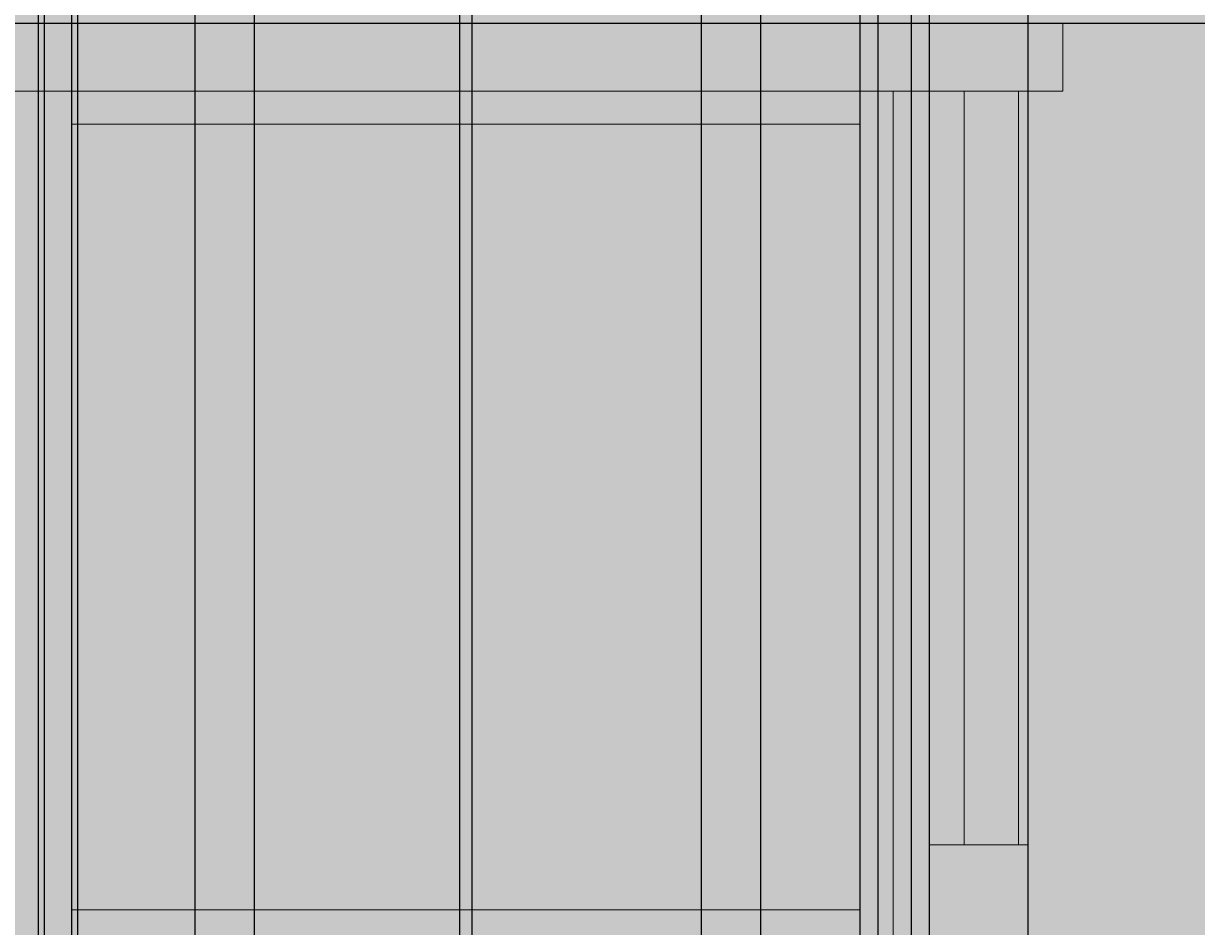
# Model space of a CAD drawing. Units: inches. Extents: x 3024 to 4744, y 1110 to 2100.
# Tile 9 of 29: x 3168 to 3309, y 1293 to 1402. Entities that reach past the tile are written whole.
import ezdxf

# ---------------------------------------------------------------- set-up
doc = ezdxf.new("R2010")
doc.units = ezdxf.units.IN
for name, color, linetype, lineweight in [('A-ANNO-DIMS', 2, 'Continuous', 18), ('A-ELEV', 7, 'Continuous', 25), ('A-ELEV-PATT', 252, 'Continuous', 13), ('A-GLAZ', 4, 'Continuous', 18)]:
    doc.layers.add(name, color=color, linetype=linetype, lineweight=lineweight)
doc.styles.get("Standard").update_dxf_attribs({"font": 'arial.ttf'})
doc.dimstyles.get("Standard").update_dxf_attribs({"dimtxt": 0.18, "dimasz": 0.18, "dimexe": 0.18, "dimexo": 0.0625, "dimgap": 0.09, "dimtad": 0, "dimtih": 1, "dimtoh": 1, "dimdec": 1, "dimzin": 0, "dimdsep": 46, "dimlunit": 3, "dimtxsty": 'Standard', "dimcen": 0.09, "dimadec": 0, "dimazin": 0, "dimtfac": 1, "dimtdec": 1, "dimtofl": 0, "dimtmove": 0, "dimatfit": 3, "dimfxl": 1, "dimtolj": 1, "dimtzin": 0, "dimarcsym": 0})

# ---------------------------------------------------------------- blocks, each defined once
blk = doc.blocks.new('WIN-BALCONY-A')
for q in [(3148.97, 1897.49), (3148.97, 1897.49), (3292.61, 1897.49), (3292.61, 1897.49)]:
    blk.add_line((3169.4, 1897.49), q)
blk.add_lwpolyline([(3148.97, 1897.49), (3148.97, 1905.61), (3292.61, 1905.61), (3292.61, 1897.49)])
blk.add_lwpolyline([(3148.97, 1897.49), (3148.97, 1905.61), (3292.61, 1905.61), (3292.61, 1897.49)])
for points in [[(3272.18, 1795.04), (3169.4, 1795.04), (3169.4, 1897.49), (3272.18, 1897.49)], [(3272.18, 1795.04), (3169.4, 1795.04), (3169.4, 1897.49), (3272.18, 1897.49)], [(3287.25, 1806.87), (3280.72, 1806.87), (3280.72, 1897.49), (3287.25, 1897.49)], [(3287.25, 1806.87), (3280.72, 1806.87), (3280.72, 1897.49), (3287.25, 1897.49)], [(3268.18, 1799.04), (3173.4, 1799.04), (3173.4, 1893.49), (3268.18, 1893.49)], [(3268.18, 1799.04), (3173.4, 1799.04), (3173.4, 1893.49), (3268.18, 1893.49)], [(3220.05, 1893.49), (3221.52, 1893.49), (3221.52, 1799.04), (3220.05, 1799.04)], [(3220.05, 1893.49), (3221.52, 1893.49), (3221.52, 1799.04), (3220.05, 1799.04)], [(3276.51, 1795.04), (3288.38, 1795.04), (3288.38, 1806.87), (3276.51, 1806.87)], [(3276.51, 1795.04), (3288.38, 1795.04), (3288.38, 1806.87), (3276.51, 1806.87)]]:
    blk.add_lwpolyline(points, close=True)
blk = doc.blocks.new('*D64')
at = {"layer": 'A-ANNO-DIMS', "color": 0, "lineweight": -2, "transparency": 16777216}
for p, q in [((3069.79, 1241.5), (3069.79, 2100.44)), ((3069.97, 2100.26), (3405.08, 2100.26)), ((3740.97, 2100.26), (3405.87, 2100.26)), ((3741.15, 1241.5), (3741.15, 2100.44))]:
    blk.add_line(p, q, dxfattribs=at)
at = {"layer": 'A-ANNO-DIMS', "color": 0, "transparency": 16777216}
for points in [[(3069.97, 2100.29), (3069.97, 2100.23), (3069.79, 2100.26)], [(3740.97, 2100.29), (3740.97, 2100.23), (3741.15, 2100.26)]]:
    blk.add_solid(points, dxfattribs=at)
at = {"layer": 'Defpoints', "color": 0, "transparency": 16777216}
for p in [(3741.15, 2100.26), (3069.79, 1241.43), (3741.15, 1241.43)]:
    blk.add_point(p, dxfattribs=at)
at = {"layer": 'A-ANNO-DIMS', "color": 0, "transparency": 16777216, "insert": (3405.47, 2100.26), "char_height": 0.18, "attachment_point": 5}
blk.add_mtext('\\A1;671.4', dxfattribs=at)
blk = doc.blocks.new('*D90')
at = {"layer": 'A-ANNO-DIMS', "color": 0, "lineweight": -2, "transparency": 16777216}
for p, q in [((3173.4, 1798.98), (3173.4, 1109.93)), ((3169.4, 1794.98), (3169.4, 1109.93)), ((3169.58, 1110.11), (3171.07, 1110.11)), ((3173.22, 1110.11), (3171.72, 1110.11))]:
    blk.add_line(p, q, dxfattribs=at)
at = {"layer": 'A-ANNO-DIMS', "color": 0, "transparency": 16777216}
for points in [[(3169.58, 1110.14), (3169.58, 1110.08), (3169.4, 1110.11)], [(3173.22, 1110.14), (3173.22, 1110.08), (3173.4, 1110.11)]]:
    blk.add_solid(points, dxfattribs=at)
at = {"layer": 'Defpoints', "color": 0, "transparency": 16777216}
for p in [(3173.4, 1799.04), (3169.4, 1795.04), (3173.4, 1110.11)]:
    blk.add_point(p, dxfattribs=at)
at = {"layer": 'A-ANNO-DIMS', "color": 0, "transparency": 16777216, "insert": (3171.4, 1110.11), "char_height": 0.18, "attachment_point": 5}
blk.add_mtext('\\A1;4.00', dxfattribs=at)
blk = doc.blocks.new('*D91')
at = {"layer": 'A-ANNO-DIMS', "color": 0, "lineweight": -2, "transparency": 16777216}
for p, q in [((3173.4, 1798.98), (3173.4, 1109.93)), ((3220.05, 1798.98), (3220.05, 1109.93)), ((3173.58, 1110.11), (3196.33, 1110.11)), ((3219.87, 1110.11), (3197.12, 1110.11))]:
    blk.add_line(p, q, dxfattribs=at)
at = {"layer": 'A-ANNO-DIMS', "color": 0, "transparency": 16777216}
for points in [[(3173.58, 1110.14), (3173.58, 1110.08), (3173.4, 1110.11)], [(3219.87, 1110.14), (3219.87, 1110.08), (3220.05, 1110.11)]]:
    blk.add_solid(points, dxfattribs=at)
at = {"layer": 'Defpoints', "color": 0, "transparency": 16777216}
for p in [(3173.4, 1799.04), (3220.05, 1799.04), (3220.05, 1110.11)]:
    blk.add_point(p, dxfattribs=at)
at = {"layer": 'A-ANNO-DIMS', "color": 0, "transparency": 16777216, "insert": (3196.72, 1110.11), "char_height": 0.18, "attachment_point": 5}
blk.add_mtext('\\A1;46.65', dxfattribs=at)
blk = doc.blocks.new('*D92')
at = {"layer": 'A-ANNO-DIMS', "color": 0, "lineweight": -2, "transparency": 16777216}
for p, q in [((3220.05, 1798.98), (3220.05, 1109.93)), ((3221.52, 1798.98), (3221.52, 1109.93)), ((3220.23, 1110.11), (3220.47, 1110.11)), ((3221.34, 1110.11), (3221.1, 1110.11))]:
    blk.add_line(p, q, dxfattribs=at)
at = {"layer": 'A-ANNO-DIMS', "color": 0, "transparency": 16777216}
for points in [[(3220.23, 1110.14), (3220.23, 1110.08), (3220.05, 1110.11)], [(3221.34, 1110.14), (3221.34, 1110.08), (3221.52, 1110.11)]]:
    blk.add_solid(points, dxfattribs=at)
at = {"layer": 'Defpoints', "color": 0, "transparency": 16777216}
for p in [(3220.05, 1799.04), (3221.52, 1799.04), (3221.52, 1110.11)]:
    blk.add_point(p, dxfattribs=at)
at = {"layer": 'A-ANNO-DIMS', "color": 0, "transparency": 16777216, "insert": (3220.79, 1110.11), "char_height": 0.18, "attachment_point": 5}
blk.add_mtext('\\A1;1.47', dxfattribs=at)
blk = doc.blocks.new('*D93')
at = {"layer": 'A-ANNO-DIMS', "color": 0, "lineweight": -2, "transparency": 16777216}
for p, q in [((3221.52, 1798.98), (3221.52, 1109.93)), ((3268.18, 1798.98), (3268.18, 1109.93)), ((3221.7, 1110.11), (3244.45, 1110.11)), ((3268, 1110.11), (3245.25, 1110.11))]:
    blk.add_line(p, q, dxfattribs=at)
at = {"layer": 'A-ANNO-DIMS', "color": 0, "transparency": 16777216}
for points in [[(3221.7, 1110.14), (3221.7, 1110.08), (3221.52, 1110.11)], [(3268, 1110.14), (3268, 1110.08), (3268.18, 1110.11)]]:
    blk.add_solid(points, dxfattribs=at)
at = {"layer": 'Defpoints', "color": 0, "transparency": 16777216}
for p in [(3221.52, 1799.04), (3268.18, 1799.04), (3268.18, 1110.11)]:
    blk.add_point(p, dxfattribs=at)
at = {"layer": 'A-ANNO-DIMS', "color": 0, "transparency": 16777216, "insert": (3244.85, 1110.11), "char_height": 0.18, "attachment_point": 5}
blk.add_mtext('\\A1;46.65', dxfattribs=at)
blk = doc.blocks.new('*D94')
at = {"layer": 'A-ANNO-DIMS', "color": 0, "lineweight": -2, "transparency": 16777216}
for p, q in [((3276.51, 1794.98), (3276.51, 1109.93)), ((3288.38, 1794.98), (3288.38, 1109.93)), ((3276.69, 1110.11), (3281.99, 1110.11)), ((3288.2, 1110.11), (3282.9, 1110.11))]:
    blk.add_line(p, q, dxfattribs=at)
at = {"layer": 'A-ANNO-DIMS', "color": 0, "transparency": 16777216}
for points in [[(3276.69, 1110.14), (3276.69, 1110.08), (3276.51, 1110.11)], [(3288.2, 1110.14), (3288.2, 1110.08), (3288.38, 1110.11)]]:
    blk.add_solid(points, dxfattribs=at)
at = {"layer": 'Defpoints', "color": 0, "transparency": 16777216}
for p in [(3276.51, 1795.04), (3288.38, 1795.04), (3288.38, 1110.11)]:
    blk.add_point(p, dxfattribs=at)
at = {"layer": 'A-ANNO-DIMS', "color": 0, "transparency": 16777216, "insert": (3282.44, 1110.11), "char_height": 0.18, "attachment_point": 5}
blk.add_mtext('\\A1;11.866', dxfattribs=at)
blk = doc.blocks.new('*D106')
at = {"layer": 'A-ANNO-DIMS', "color": 0, "lineweight": -2, "transparency": 16777216}
for p, q in [((3170.16, 1275.67), (3170.16, 2100.44)), ((3170.34, 2100.26), (3171.83, 2100.26)), ((3173.98, 2100.26), (3172.49, 2100.26)), ((3174.16, 1271.67), (3174.16, 2100.44))]:
    blk.add_line(p, q, dxfattribs=at)
at = {"layer": 'A-ANNO-DIMS', "color": 0, "transparency": 16777216}
for points in [[(3170.34, 2100.29), (3170.34, 2100.23), (3170.16, 2100.26)], [(3173.98, 2100.29), (3173.98, 2100.23), (3174.16, 2100.26)]]:
    blk.add_solid(points, dxfattribs=at)
at = {"layer": 'Defpoints', "color": 0, "transparency": 16777216}
for p in [(3174.16, 2100.26), (3170.16, 1275.61), (3174.16, 1271.61)]:
    blk.add_point(p, dxfattribs=at)
at = {"layer": 'A-ANNO-DIMS', "color": 0, "transparency": 16777216, "insert": (3172.16, 2100.26), "char_height": 0.18, "attachment_point": 5}
blk.add_mtext('\\A1;4.00', dxfattribs=at)
blk = doc.blocks.new('*D107')
at = {"layer": 'A-ANNO-DIMS', "color": 0, "lineweight": -2, "transparency": 16777216}
for p, q in [((3174.16, 1271.67), (3174.16, 2100.44)), ((3174.34, 2100.26), (3221.88, 2100.26)), ((3270.21, 2100.26), (3222.67, 2100.26)), ((3270.39, 1271.67), (3270.39, 2100.44))]:
    blk.add_line(p, q, dxfattribs=at)
at = {"layer": 'A-ANNO-DIMS', "color": 0, "transparency": 16777216}
for points in [[(3174.34, 2100.29), (3174.34, 2100.23), (3174.16, 2100.26)], [(3270.21, 2100.29), (3270.21, 2100.23), (3270.39, 2100.26)]]:
    blk.add_solid(points, dxfattribs=at)
at = {"layer": 'Defpoints', "color": 0, "transparency": 16777216}
for p in [(3270.39, 2100.26), (3174.16, 1271.61), (3270.39, 1271.61)]:
    blk.add_point(p, dxfattribs=at)
at = {"layer": 'A-ANNO-DIMS', "color": 0, "transparency": 16777216, "insert": (3222.27, 2100.26), "char_height": 0.18, "attachment_point": 5}
blk.add_mtext('\\A1;96.23', dxfattribs=at)
blk = doc.blocks.new('*D108')
at = {"layer": 'A-ANNO-DIMS', "color": 0, "lineweight": -2, "transparency": 16777216}
for p, q in [((3270.39, 1271.67), (3270.39, 2100.44)), ((3270.57, 2100.26), (3272.06, 2100.26)), ((3274.21, 2100.26), (3272.71, 2100.26)), ((3274.39, 1275.67), (3274.39, 2100.44))]:
    blk.add_line(p, q, dxfattribs=at)
at = {"layer": 'A-ANNO-DIMS', "color": 0, "transparency": 16777216}
for points in [[(3270.57, 2100.29), (3270.57, 2100.23), (3270.39, 2100.26)], [(3274.21, 2100.29), (3274.21, 2100.23), (3274.39, 2100.26)]]:
    blk.add_solid(points, dxfattribs=at)
at = {"layer": 'Defpoints', "color": 0, "transparency": 16777216}
for p in [(3274.39, 2100.26), (3274.39, 1275.61), (3270.39, 1271.61)]:
    blk.add_point(p, dxfattribs=at)
at = {"layer": 'A-ANNO-DIMS', "color": 0, "transparency": 16777216, "insert": (3272.39, 2100.26), "char_height": 0.18, "attachment_point": 5}
blk.add_mtext('\\A1;4.00', dxfattribs=at)
blk = doc.blocks.new('*D124')
at = {"layer": 'A-ANNO-DIMS', "color": 0, "lineweight": -2, "transparency": 16777216}
for p, q in [((3174.16, 1271.67), (3174.16, 2100.44)), ((3174.34, 2100.26), (3180.75, 2100.26)), ((3188.08, 2100.26), (3181.67, 2100.26)), ((3188.26, 1256.29), (3188.26, 2100.44))]:
    blk.add_line(p, q, dxfattribs=at)
at = {"layer": 'A-ANNO-DIMS', "color": 0, "transparency": 16777216}
for points in [[(3174.34, 2100.29), (3174.34, 2100.23), (3174.16, 2100.26)], [(3188.08, 2100.29), (3188.08, 2100.23), (3188.26, 2100.26)]]:
    blk.add_solid(points, dxfattribs=at)
at = {"layer": 'Defpoints', "color": 0, "transparency": 16777216}
for p in [(3188.26, 2100.26), (3174.16, 1271.61), (3188.26, 1256.23)]:
    blk.add_point(p, dxfattribs=at)
at = {"layer": 'A-ANNO-DIMS', "color": 0, "transparency": 16777216, "insert": (3181.21, 2100.26), "char_height": 0.18, "attachment_point": 5}
blk.add_mtext('\\A1;14.098', dxfattribs=at)
blk = doc.blocks.new('*D125')
at = {"layer": 'A-ANNO-DIMS', "color": 0, "lineweight": -2, "transparency": 16777216}
for p, q in [((3188.26, 1256.29), (3188.26, 2100.44)), ((3188.44, 2100.26), (3191.44, 2100.26)), ((3195.23, 2100.26), (3192.22, 2100.26)), ((3195.41, 1256.29), (3195.41, 2100.44))]:
    blk.add_line(p, q, dxfattribs=at)
at = {"layer": 'A-ANNO-DIMS', "color": 0, "transparency": 16777216}
for points in [[(3188.44, 2100.29), (3188.44, 2100.23), (3188.26, 2100.26)], [(3195.23, 2100.29), (3195.23, 2100.23), (3195.41, 2100.26)]]:
    blk.add_solid(points, dxfattribs=at)
at = {"layer": 'Defpoints', "color": 0, "transparency": 16777216}
for p in [(3195.41, 2100.26), (3188.26, 1256.23), (3195.41, 1256.23)]:
    blk.add_point(p, dxfattribs=at)
at = {"layer": 'A-ANNO-DIMS', "color": 0, "transparency": 16777216, "insert": (3191.83, 2100.26), "char_height": 0.18, "attachment_point": 5}
blk.add_mtext('\\A1;7.147', dxfattribs=at)
blk = doc.blocks.new('*D126')
at = {"layer": 'A-ANNO-DIMS', "color": 0, "lineweight": -2, "transparency": 16777216}
for p, q in [((3249.14, 1256.29), (3249.14, 2100.44)), ((3249.32, 2100.26), (3252.32, 2100.26)), ((3256.11, 2100.26), (3253.11, 2100.26)), ((3256.29, 1256.29), (3256.29, 2100.44))]:
    blk.add_line(p, q, dxfattribs=at)
at = {"layer": 'A-ANNO-DIMS', "color": 0, "transparency": 16777216}
for points in [[(3249.32, 2100.29), (3249.32, 2100.23), (3249.14, 2100.26)], [(3256.11, 2100.29), (3256.11, 2100.23), (3256.29, 2100.26)]]:
    blk.add_solid(points, dxfattribs=at)
at = {"layer": 'Defpoints', "color": 0, "transparency": 16777216}
for p in [(3256.29, 2100.26), (3249.14, 1256.23), (3256.29, 1256.23)]:
    blk.add_point(p, dxfattribs=at)
at = {"layer": 'A-ANNO-DIMS', "color": 0, "transparency": 16777216, "insert": (3252.72, 2100.26), "char_height": 0.18, "attachment_point": 5}
blk.add_mtext('\\A1;7.147', dxfattribs=at)

msp = doc.modelspace()

# ---------------------------------------------------------------- hatches: boundary and pattern name
at = {"layer": 'A-ELEV-PATT'}
h = msp.add_hatch(color=256, dxfattribs=at)
h.dxf.hatch_style = 1
h.paths.add_polyline_path([(3491.8271, 2054.7584), (3320.5658, 2054.7584), (3320.5658, 2043.5286), (3491.8271, 2043.5286)])
h.paths.add_polyline_path([(3292.6051, 1905.6112), (3148.9694, 1905.6112), (3148.9694, 1897.4879), (3169.3964, 1897.4879), (3292.6051, 1897.4879)])
h.paths.add_polyline_path([(3292.6051, 1795.0431), (3169.3964, 1795.0431), (3148.9694, 1795.0431), (3148.9694, 1785.6112), (3292.6051, 1785.6112)])
h.paths.add_polyline_path([(3292.6051, 1779.6112), (3148.9694, 1779.6112), (3148.9694, 1771.4879), (3169.3964, 1771.4879), (3292.6051, 1771.4879)])
h.paths.add_polyline_path([(3292.6051, 1669.0431), (3169.3964, 1669.0431), (3148.9694, 1669.0431), (3148.9694, 1659.6112), (3292.6051, 1659.6112)])
h.paths.add_polyline_path([(3292.6051, 1653.6112), (3148.9694, 1653.6112), (3148.9694, 1645.4879), (3169.3964, 1645.4879), (3292.6051, 1645.4879)])
h.paths.add_polyline_path([(3292.6051, 1543.0431), (3169.3964, 1543.0431), (3148.9694, 1543.0431), (3148.9694, 1533.6112), (3292.6051, 1533.6112)])
h.paths.add_polyline_path([(3292.6051, 1527.6112), (3148.9694, 1527.6112), (3148.9694, 1519.4879), (3169.3964, 1519.4879), (3292.6051, 1519.4879)])
h.paths.add_polyline_path([(3292.6051, 1401.6112), (3148.9694, 1401.6112), (3148.9694, 1393.4879), (3169.3964, 1393.4879), (3292.6051, 1393.4879)])
h.paths.add_polyline_path([(3292.6051, 1417.0431), (3169.3964, 1417.0431), (3148.9694, 1417.0431), (3148.9694, 1407.6112), (3292.6051, 1407.6112)])
h.paths.add_polyline_path([(3292.6051, 1291.0431), (3169.3964, 1291.0431), (3148.9694, 1291.0431), (3148.9694, 1281.6112), (3292.6051, 1281.6112)])
h.paths.add_polyline_path([(3654.037, 1165.0431), (3530.8283, 1165.0431), (3510.4013, 1165.0431), (3510.4013, 1155.6112), (3654.037, 1155.6112)])
h.paths.add_polyline_path([(3654.037, 1275.6112), (3510.4013, 1275.6112), (3510.4013, 1267.4879), (3530.8283, 1267.4879), (3654.037, 1267.4879)])
h.paths.add_polyline_path([(3654.037, 1291.0431), (3530.8283, 1291.0431), (3510.4013, 1291.0431), (3510.4013, 1281.6112), (3654.037, 1281.6112)])
h.paths.add_polyline_path([(3654.037, 1417.0431), (3530.8283, 1417.0431), (3510.4013, 1417.0431), (3510.4013, 1407.6112), (3654.037, 1407.6112)])
h.paths.add_polyline_path([(3654.037, 1401.6112), (3510.4013, 1401.6112), (3510.4013, 1393.4879), (3530.8283, 1393.4879), (3654.037, 1393.4879)])
h.paths.add_polyline_path([(3654.037, 1543.0431), (3530.8283, 1543.0431), (3510.4013, 1543.0431), (3510.4013, 1533.6112), (3654.037, 1533.6112)])
h.paths.add_polyline_path([(3654.037, 1527.6112), (3510.4013, 1527.6112), (3510.4013, 1519.4879), (3530.8283, 1519.4879), (3654.037, 1519.4879)])
h.paths.add_polyline_path([(3654.037, 1653.6112), (3510.4013, 1653.6112), (3510.4013, 1645.4879), (3530.8283, 1645.4879), (3654.037, 1645.4879)])
h.paths.add_polyline_path([(3654.037, 1669.0431), (3530.8283, 1669.0431), (3510.4013, 1669.0431), (3510.4013, 1659.6112), (3654.037, 1659.6112)])
h.paths.add_polyline_path([(3654.037, 1779.6112), (3510.4013, 1779.6112), (3510.4013, 1771.4879), (3530.8283, 1771.4879), (3654.037, 1771.4879)])
h.paths.add_polyline_path([(3654.037, 1795.0431), (3530.8283, 1795.0431), (3510.4013, 1795.0431), (3510.4013, 1785.6112), (3654.037, 1785.6112)])
h.paths.add_polyline_path([(3654.037, 1905.6112), (3510.4013, 1905.6112), (3510.4013, 1897.4879), (3530.8283, 1897.4879), (3654.037, 1897.4879)])
h = msp.add_hatch(color=256, dxfattribs=at)
h.dxf.hatch_style = 1
h.paths.add_polyline_path([(3329.7033, 1407.6112), (3105.4722, 1407.6112), (3105.4722, 1401.6112), (3329.7033, 1401.6112)])
h.paths.add_polyline_path([(3329.7033, 1281.6112), (3105.4722, 1281.6112), (3105.4722, 1275.6112), (3112.3838, 1275.6112), (3329.7033, 1275.6112)])
h.paths.add_polyline_path([(3329.7033, 1533.6112), (3105.4722, 1533.6112), (3105.4722, 1527.6112), (3329.7033, 1527.6112)])
h.paths.add_polyline_path([(3329.7033, 1659.6112), (3105.4722, 1659.6112), (3105.4722, 1653.6112), (3329.7033, 1653.6112)])
h.paths.add_polyline_path([(3329.7033, 1785.6112), (3105.4722, 1785.6112), (3105.4722, 1779.6112), (3329.7033, 1779.6112)])
h.paths.add_polyline_path([(3329.7033, 1911.6112), (3105.4722, 1911.6112), (3095.7158, 1911.6112), (3095.7158, 1905.6112), (3329.7033, 1905.6112)])
h.paths.add_polyline_path([(3715.2286, 1911.6112), (3705.4722, 1911.6112), (3705.4722, 1905.6112), (3715.2286, 1905.6112)])
h.paths.add_polyline_path([(3688.5588, 1911.6112), (3481.2411, 1911.6112), (3481.2411, 1905.6112), (3688.5588, 1905.6112)])
h = msp.add_hatch(color=256, dxfattribs=at)
h.dxf.hatch_style = 1
h.paths.add_polyline_path([(3154.3287, 1897.4879), (3148.9694, 1897.4879), (3148.9694, 1905.6112), (3105.4722, 1905.6112), (3105.4722, 1785.6112), (3148.9694, 1785.6112), (3148.9694, 1795.0431), (3151.6604, 1795.0431), (3151.6604, 1806.8674), (3154.3287, 1806.8674)])
h.paths.add_polyline_path([(3329.7033, 1905.6112), (3292.6051, 1905.6112), (3292.6051, 1897.4879), (3287.2458, 1897.4879), (3287.2458, 1806.8674), (3288.3759, 1806.8674), (3288.3759, 1795.0431), (3292.6051, 1795.0431), (3292.6051, 1785.6112), (3329.7033, 1785.6112)])
h.paths.add_polyline_path([(3154.3287, 1771.4879), (3148.9694, 1771.4879), (3148.9694, 1779.6112), (3105.4722, 1779.6112), (3105.4722, 1659.6112), (3148.9694, 1659.6112), (3148.9694, 1669.0431), (3151.6604, 1669.0431), (3151.6604, 1680.8674), (3154.3287, 1680.8674)])
h.paths.add_polyline_path([(3329.7033, 1779.6112), (3292.6051, 1779.6112), (3292.6051, 1771.4879), (3287.2458, 1771.4879), (3287.2458, 1680.8674), (3288.3759, 1680.8674), (3288.3759, 1669.0431), (3292.6051, 1669.0431), (3292.6051, 1659.6112), (3329.7033, 1659.6112)])
h.paths.add_polyline_path([(3154.3287, 1645.4879), (3148.9694, 1645.4879), (3148.9694, 1653.6112), (3105.4722, 1653.6112), (3105.4722, 1533.6112), (3148.9694, 1533.6112), (3148.9694, 1543.0431), (3151.6604, 1543.0431), (3151.6604, 1554.8674), (3154.3287, 1554.8674)])
h.paths.add_polyline_path([(3329.7033, 1653.6112), (3292.6051, 1653.6112), (3292.6051, 1645.4879), (3287.2458, 1645.4879), (3287.2458, 1554.8674), (3288.3759, 1554.8674), (3288.3759, 1543.0431), (3292.6051, 1543.0431), (3292.6051, 1533.6112), (3329.7033, 1533.6112)])
h.paths.add_polyline_path([(3329.7033, 1527.6112), (3292.6051, 1527.6112), (3292.6051, 1519.4879), (3287.2458, 1519.4879), (3287.2458, 1428.8674), (3288.3759, 1428.8674), (3288.3759, 1417.0431), (3292.6051, 1417.0431), (3292.6051, 1407.6112), (3329.7033, 1407.6112)])
h.paths.add_polyline_path([(3329.7033, 1401.6112), (3292.6051, 1401.6112), (3292.6051, 1393.4879), (3287.2458, 1393.4879), (3287.2458, 1302.8674), (3288.3759, 1302.8674), (3288.3759, 1291.0431), (3292.6051, 1291.0431), (3292.6051, 1281.6112), (3329.7033, 1281.6112)])
h.paths.add_polyline_path([(3154.3287, 1393.4879), (3148.9694, 1393.4879), (3148.9694, 1401.6112), (3105.4722, 1401.6112), (3105.4722, 1281.6112), (3148.9694, 1281.6112), (3148.9694, 1291.0431), (3151.6604, 1291.0431), (3151.6604, 1302.8674), (3154.3287, 1302.8674)])
h.paths.add_polyline_path([(3154.3287, 1519.4879), (3148.9694, 1519.4879), (3148.9694, 1527.6112), (3105.4722, 1527.6112), (3105.4722, 1407.6112), (3148.9694, 1407.6112), (3148.9694, 1417.0431), (3151.6604, 1417.0431), (3151.6604, 1428.8674), (3154.3287, 1428.8674)])
h.paths.add_polyline_path([(3515.7606, 1897.4879), (3510.4013, 1897.4879), (3510.4013, 1905.6112), (3481.2411, 1905.6112), (3481.2411, 1785.6112), (3510.4013, 1785.6112), (3510.4013, 1795.0431), (3513.0923, 1795.0431), (3513.0923, 1806.8674), (3515.7606, 1806.8674)])
h.paths.add_polyline_path([(3688.5588, 1905.6112), (3654.037, 1905.6112), (3654.037, 1897.4879), (3648.6777, 1897.4879), (3648.6777, 1806.8674), (3649.8078, 1806.8674), (3649.8078, 1795.0431), (3654.037, 1795.0431), (3654.037, 1785.6112), (3688.5588, 1785.6112)])
h.paths.add_polyline_path([(3515.7606, 1771.4879), (3510.4013, 1771.4879), (3510.4013, 1779.6112), (3481.2411, 1779.6112), (3481.2411, 1659.6112), (3510.4013, 1659.6112), (3510.4013, 1669.0431), (3513.0923, 1669.0431), (3513.0923, 1680.8674), (3515.7606, 1680.8674)])
h.paths.add_polyline_path([(3688.5588, 1779.6112), (3654.037, 1779.6112), (3654.037, 1771.4879), (3648.6777, 1771.4879), (3648.6777, 1680.8674), (3649.8078, 1680.8674), (3649.8078, 1669.0431), (3654.037, 1669.0431), (3654.037, 1659.6112), (3688.5588, 1659.6112)])
h.paths.add_polyline_path([(3515.7606, 1645.4879), (3510.4013, 1645.4879), (3510.4013, 1653.6112), (3481.2411, 1653.6112), (3481.2411, 1533.6112), (3510.4013, 1533.6112), (3510.4013, 1543.0431), (3513.0923, 1543.0431), (3513.0923, 1554.8674), (3515.7606, 1554.8674)])
h.paths.add_polyline_path([(3688.5588, 1653.6112), (3654.037, 1653.6112), (3654.037, 1645.4879), (3648.6777, 1645.4879), (3648.6777, 1554.8674), (3649.8078, 1554.8674), (3649.8078, 1543.0431), (3654.037, 1543.0431), (3654.037, 1533.6112), (3688.5588, 1533.6112)])
h.paths.add_polyline_path([(3515.7606, 1519.4879), (3510.4013, 1519.4879), (3510.4013, 1527.6112), (3481.2411, 1527.6112), (3481.2411, 1407.6112), (3510.4013, 1407.6112), (3510.4013, 1417.0431), (3513.0923, 1417.0431), (3513.0923, 1428.8674), (3515.7606, 1428.8674)])
h.paths.add_polyline_path([(3688.5588, 1527.6112), (3654.037, 1527.6112), (3654.037, 1519.4879), (3648.6777, 1519.4879), (3648.6777, 1428.8674), (3649.8078, 1428.8674), (3649.8078, 1417.0431), (3654.037, 1417.0431), (3654.037, 1407.6112), (3688.5588, 1407.6112)])
h.paths.add_polyline_path([(3515.7606, 1393.4879), (3510.4013, 1393.4879), (3510.4013, 1401.6112), (3481.2411, 1401.6112), (3481.2411, 1281.6112), (3510.4013, 1281.6112), (3510.4013, 1291.0431), (3513.0923, 1291.0431), (3513.0923, 1302.8674), (3515.7606, 1302.8674)])
h.paths.add_polyline_path([(3688.5588, 1401.6112), (3654.037, 1401.6112), (3654.037, 1393.4879), (3648.6777, 1393.4879), (3648.6777, 1302.8674), (3649.8078, 1302.8674), (3649.8078, 1291.0431), (3654.037, 1291.0431), (3654.037, 1281.6112), (3688.5588, 1281.6112)])
h.paths.add_polyline_path([(3515.7606, 1267.4879), (3510.4013, 1267.4879), (3510.4013, 1275.6112), (3481.2411, 1275.6112), (3481.2411, 1155.6112), (3510.4013, 1155.6112), (3510.4013, 1165.0431), (3513.0923, 1165.0431), (3513.0923, 1176.8674), (3515.7606, 1176.8674)])
h.paths.add_polyline_path([(3688.5588, 1275.6112), (3654.037, 1275.6112), (3654.037, 1267.4879), (3648.6777, 1267.4879), (3648.6777, 1176.8674), (3649.8078, 1176.8674), (3649.8078, 1165.0431), (3654.037, 1165.0431), (3654.037, 1155.6112), (3688.5588, 1155.6112)])
h.paths.add_polyline_path([(3112.3838, 1275.6112), (3105.4722, 1275.6112), (3105.4722, 1171.0239), (3112.3838, 1171.0239)])
h = msp.add_hatch(color=256, dxfattribs=at)
h.dxf.hatch_style = 1
h.paths.add_polyline_path([(3160.8586, 1897.4879), (3154.3287, 1897.4879), (3154.3287, 1806.8674), (3160.8586, 1806.8674)])
h.paths.add_polyline_path([(3287.2458, 1897.4879), (3280.716, 1897.4879), (3280.716, 1806.8674), (3287.2458, 1806.8674)])
h.paths.add_polyline_path([(3160.8586, 1771.4879), (3154.3287, 1771.4879), (3154.3287, 1680.8674), (3160.8586, 1680.8674)])
h.paths.add_polyline_path([(3287.2458, 1771.4879), (3280.716, 1771.4879), (3280.716, 1680.8674), (3287.2458, 1680.8674)])
h.paths.add_polyline_path([(3160.8586, 1645.4879), (3154.3287, 1645.4879), (3154.3287, 1554.8674), (3160.8586, 1554.8674)])
h.paths.add_polyline_path([(3287.2458, 1645.4879), (3280.716, 1645.4879), (3280.716, 1554.8674), (3287.2458, 1554.8674)])
h.paths.add_polyline_path([(3160.8586, 1519.4879), (3154.3287, 1519.4879), (3154.3287, 1428.8674), (3160.8586, 1428.8674)])
h.paths.add_polyline_path([(3287.2458, 1519.4879), (3280.716, 1519.4879), (3280.716, 1428.8674), (3287.2458, 1428.8674)])
h.paths.add_polyline_path([(3160.8586, 1393.4879), (3154.3287, 1393.4879), (3154.3287, 1302.8674), (3160.8586, 1302.8674)])
h.paths.add_polyline_path([(3287.2458, 1393.4879), (3280.716, 1393.4879), (3280.716, 1302.8674), (3287.2458, 1302.8674)])
h.paths.add_polyline_path([(3648.6777, 1267.4879), (3642.1479, 1267.4879), (3642.1479, 1176.8674), (3648.6777, 1176.8674)])
h.paths.add_polyline_path([(3522.2905, 1267.4879), (3515.7606, 1267.4879), (3515.7606, 1176.8674), (3522.2905, 1176.8674)])
h.paths.add_polyline_path([(3522.2905, 1393.4879), (3515.7606, 1393.4879), (3515.7606, 1302.8674), (3522.2905, 1302.8674)])
h.paths.add_polyline_path([(3648.6777, 1393.4879), (3642.1479, 1393.4879), (3642.1479, 1302.8674), (3648.6777, 1302.8674)])
h.paths.add_polyline_path([(3522.2905, 1519.4879), (3515.7606, 1519.4879), (3515.7606, 1428.8674), (3522.2905, 1428.8674)])
h.paths.add_polyline_path([(3648.6777, 1519.4879), (3642.1479, 1519.4879), (3642.1479, 1428.8674), (3648.6777, 1428.8674)])
h.paths.add_polyline_path([(3522.2905, 1645.4879), (3515.7606, 1645.4879), (3515.7606, 1554.8674), (3522.2905, 1554.8674)])
h.paths.add_polyline_path([(3522.2905, 1771.4879), (3515.7606, 1771.4879), (3515.7606, 1680.8674), (3522.2905, 1680.8674)])
h.paths.add_polyline_path([(3648.6777, 1645.4879), (3642.1479, 1645.4879), (3642.1479, 1554.8674), (3648.6777, 1554.8674)])
h.paths.add_polyline_path([(3648.6777, 1771.4879), (3642.1479, 1771.4879), (3642.1479, 1680.8674), (3648.6777, 1680.8674)])
h.paths.add_polyline_path([(3648.6777, 1897.4879), (3642.1479, 1897.4879), (3642.1479, 1806.8674), (3648.6777, 1806.8674)])
h.paths.add_polyline_path([(3522.2905, 1897.4879), (3515.7606, 1897.4879), (3515.7606, 1806.8674), (3522.2905, 1806.8674)])
h = msp.add_hatch(color=256, dxfattribs=at)
h.dxf.hatch_style = 1
h.paths.add_polyline_path([(3169.3964, 1897.4879), (3160.8586, 1897.4879), (3160.8586, 1806.8674), (3163.5269, 1806.8674), (3163.5269, 1795.0431), (3169.3964, 1795.0431)])
h.paths.add_polyline_path([(3280.716, 1897.4879), (3272.1781, 1897.4879), (3272.1781, 1795.0431), (3276.5094, 1795.0431), (3276.5094, 1806.8674), (3280.716, 1806.8674)])
h.paths.add_polyline_path([(3280.716, 1771.4879), (3272.1781, 1771.4879), (3272.1781, 1669.0431), (3276.5094, 1669.0431), (3276.5094, 1680.8674), (3280.716, 1680.8674)])
h.paths.add_polyline_path([(3169.3964, 1771.4879), (3160.8586, 1771.4879), (3160.8586, 1680.8674), (3163.5269, 1680.8674), (3163.5269, 1669.0431), (3169.3964, 1669.0431)])
h.paths.add_polyline_path([(3169.3964, 1645.4879), (3160.8586, 1645.4879), (3160.8586, 1554.8674), (3163.5269, 1554.8674), (3163.5269, 1543.0431), (3169.3964, 1543.0431)])
h.paths.add_polyline_path([(3280.716, 1645.4879), (3272.1781, 1645.4879), (3272.1781, 1543.0431), (3276.5094, 1543.0431), (3276.5094, 1554.8674), (3280.716, 1554.8674)])
h.paths.add_polyline_path([(3169.3964, 1519.4879), (3160.8586, 1519.4879), (3160.8586, 1428.8674), (3163.5269, 1428.8674), (3163.5269, 1417.0431), (3169.3964, 1417.0431)])
h.paths.add_polyline_path([(3280.716, 1519.4879), (3272.1781, 1519.4879), (3272.1781, 1417.0431), (3276.5094, 1417.0431), (3276.5094, 1428.8674), (3280.716, 1428.8674)])
h.paths.add_polyline_path([(3169.3964, 1393.4879), (3160.8586, 1393.4879), (3160.8586, 1302.8674), (3163.5269, 1302.8674), (3163.5269, 1291.0431), (3169.3964, 1291.0431)])
h.paths.add_polyline_path([(3280.716, 1393.4879), (3272.1781, 1393.4879), (3272.1781, 1291.0431), (3276.5094, 1291.0431), (3276.5094, 1302.8674), (3280.716, 1302.8674)])
h.paths.add_polyline_path([(3642.1479, 1267.4879), (3633.61, 1267.4879), (3633.61, 1165.0431), (3637.9413, 1165.0431), (3637.9413, 1176.8674), (3642.1479, 1176.8674)])
h.paths.add_polyline_path([(3530.8283, 1267.4879), (3522.2905, 1267.4879), (3522.2905, 1176.8674), (3524.9588, 1176.8674), (3524.9588, 1165.0431), (3530.8283, 1165.0431)])
h.paths.add_polyline_path([(3642.1479, 1393.4879), (3633.61, 1393.4879), (3633.61, 1291.0431), (3637.9413, 1291.0431), (3637.9413, 1302.8674), (3642.1479, 1302.8674)])
h.paths.add_polyline_path([(3530.8283, 1393.4879), (3522.2905, 1393.4879), (3522.2905, 1302.8674), (3524.9588, 1302.8674), (3524.9588, 1291.0431), (3530.8283, 1291.0431)])
h.paths.add_polyline_path([(3530.8283, 1519.4879), (3522.2905, 1519.4879), (3522.2905, 1428.8674), (3524.9588, 1428.8674), (3524.9588, 1417.0431), (3530.8283, 1417.0431)])
h.paths.add_polyline_path([(3642.1479, 1519.4879), (3633.61, 1519.4879), (3633.61, 1417.0431), (3637.9413, 1417.0431), (3637.9413, 1428.8674), (3642.1479, 1428.8674)])
h.paths.add_polyline_path([(3530.8283, 1645.4879), (3522.2905, 1645.4879), (3522.2905, 1554.8674), (3524.9588, 1554.8674), (3524.9588, 1543.0431), (3530.8283, 1543.0431)])
h.paths.add_polyline_path([(3642.1479, 1645.4879), (3633.61, 1645.4879), (3633.61, 1543.0431), (3637.9413, 1543.0431), (3637.9413, 1554.8674), (3642.1479, 1554.8674)])
h.paths.add_polyline_path([(3642.1479, 1771.4879), (3633.61, 1771.4879), (3633.61, 1669.0431), (3637.9413, 1669.0431), (3637.9413, 1680.8674), (3642.1479, 1680.8674)])
h.paths.add_polyline_path([(3530.8283, 1771.4879), (3522.2905, 1771.4879), (3522.2905, 1680.8674), (3524.9588, 1680.8674), (3524.9588, 1669.0431), (3530.8283, 1669.0431)])
h.paths.add_polyline_path([(3530.8283, 1897.4879), (3522.2905, 1897.4879), (3522.2905, 1806.8674), (3524.9588, 1806.8674), (3524.9588, 1795.0431), (3530.8283, 1795.0431)])
h.paths.add_polyline_path([(3642.1479, 1897.4879), (3633.61, 1897.4879), (3633.61, 1795.0431), (3637.9413, 1795.0431), (3637.9413, 1806.8674), (3642.1479, 1806.8674)])
h = msp.add_hatch(color=256, dxfattribs=at)
h.dxf.hatch_style = 1
h.paths.add_polyline_path([(3220.0505, 1893.4879), (3173.3964, 1893.4879), (3173.3964, 1799.0431), (3220.0505, 1799.0431)])
h.paths.add_polyline_path([(3268.1781, 1893.4879), (3221.5241, 1893.4879), (3221.5241, 1799.0431), (3268.1781, 1799.0431)])
h.paths.add_polyline_path([(3581.4824, 1893.4879), (3534.8283, 1893.4879), (3534.8283, 1799.0431), (3581.4824, 1799.0431)])
h.paths.add_polyline_path([(3629.61, 1893.4879), (3582.956, 1893.4879), (3582.956, 1799.0431), (3629.61, 1799.0431)])
h.paths.add_polyline_path([(3581.4824, 1767.4879), (3534.8283, 1767.4879), (3534.8283, 1673.0431), (3581.4824, 1673.0431)])
h.paths.add_polyline_path([(3629.61, 1767.4879), (3582.956, 1767.4879), (3582.956, 1673.0431), (3629.61, 1673.0431)])
h.paths.add_polyline_path([(3581.4824, 1641.4879), (3534.8283, 1641.4879), (3534.8283, 1547.0431), (3581.4824, 1547.0431)])
h.paths.add_polyline_path([(3629.61, 1641.4879), (3582.956, 1641.4879), (3582.956, 1547.0431), (3629.61, 1547.0431)])
h.paths.add_polyline_path([(3629.61, 1515.4879), (3582.956, 1515.4879), (3582.956, 1421.0431), (3629.61, 1421.0431)])
h.paths.add_polyline_path([(3581.4824, 1515.4879), (3534.8283, 1515.4879), (3534.8283, 1421.0431), (3581.4824, 1421.0431)])
h.paths.add_polyline_path([(3629.61, 1389.4879), (3582.956, 1389.4879), (3582.956, 1295.0431), (3629.61, 1295.0431)])
h.paths.add_polyline_path([(3581.4824, 1389.4879), (3534.8283, 1389.4879), (3534.8283, 1295.0431), (3581.4824, 1295.0431)])
h.paths.add_polyline_path([(3629.61, 1263.4879), (3582.956, 1263.4879), (3582.956, 1169.0431), (3629.61, 1169.0431)])
h.paths.add_polyline_path([(3581.4824, 1263.4879), (3534.8283, 1263.4879), (3534.8283, 1169.0431), (3581.4824, 1169.0431)])
h.paths.add_polyline_path([(3220.0505, 1389.4879), (3173.3964, 1389.4879), (3173.3964, 1295.0431), (3220.0505, 1295.0431)])
h.paths.add_polyline_path([(3268.1781, 1389.4879), (3221.5241, 1389.4879), (3221.5241, 1295.0431), (3268.1781, 1295.0431)])
h.paths.add_polyline_path([(3220.0505, 1515.4879), (3173.3964, 1515.4879), (3173.3964, 1421.0431), (3220.0505, 1421.0431)])
h.paths.add_polyline_path([(3268.1781, 1515.4879), (3221.5241, 1515.4879), (3221.5241, 1421.0431), (3268.1781, 1421.0431)])
h.paths.add_polyline_path([(3220.0505, 1767.4879), (3173.3964, 1767.4879), (3173.3964, 1673.0431), (3220.0505, 1673.0431)])
h.paths.add_polyline_path([(3268.1781, 1767.4879), (3221.5241, 1767.4879), (3221.5241, 1673.0431), (3268.1781, 1673.0431)])
h.paths.add_polyline_path([(3220.0505, 1641.4879), (3173.3964, 1641.4879), (3173.3964, 1547.0431), (3220.0505, 1547.0431)])
h.paths.add_polyline_path([(3268.1781, 1641.4879), (3221.5241, 1641.4879), (3221.5241, 1547.0431), (3268.1781, 1547.0431)])
h = msp.add_hatch(color=256, dxfattribs=at)
h.dxf.hatch_style = 1
h.paths.add_polyline_path([(3163.5269, 1302.8674), (3151.6604, 1302.8674), (3151.6604, 1291.0431), (3163.5269, 1291.0431)])
h.paths.add_polyline_path([(3288.3759, 1302.8674), (3276.5094, 1302.8674), (3276.5094, 1291.0431), (3288.3759, 1291.0431)])
h.paths.add_polyline_path([(3288.3759, 1428.8674), (3276.5094, 1428.8674), (3276.5094, 1417.0431), (3288.3759, 1417.0431)])
h.paths.add_polyline_path([(3163.5269, 1428.8674), (3151.6604, 1428.8674), (3151.6604, 1417.0431), (3163.5269, 1417.0431)])
h.paths.add_polyline_path([(3163.5269, 1554.8674), (3151.6604, 1554.8674), (3151.6604, 1543.0431), (3163.5269, 1543.0431)])
h.paths.add_polyline_path([(3288.3759, 1554.8674), (3276.5094, 1554.8674), (3276.5094, 1543.0431), (3288.3759, 1543.0431)])
h.paths.add_polyline_path([(3163.5269, 1680.8674), (3151.6604, 1680.8674), (3151.6604, 1669.0431), (3163.5269, 1669.0431)])
h.paths.add_polyline_path([(3288.3759, 1680.8674), (3276.5094, 1680.8674), (3276.5094, 1669.0431), (3288.3759, 1669.0431)])
h.paths.add_polyline_path([(3163.5269, 1806.8674), (3151.6604, 1806.8674), (3151.6604, 1795.0431), (3163.5269, 1795.0431)])
h.paths.add_polyline_path([(3288.3759, 1806.8674), (3276.5094, 1806.8674), (3276.5094, 1795.0431), (3288.3759, 1795.0431)])
h.paths.add_polyline_path([(3524.9588, 1806.8674), (3513.0923, 1806.8674), (3513.0923, 1795.0431), (3524.9588, 1795.0431)])
h.paths.add_polyline_path([(3649.8078, 1806.8674), (3637.9413, 1806.8674), (3637.9413, 1795.0431), (3649.8078, 1795.0431)])
h.paths.add_polyline_path([(3524.9588, 1680.8674), (3513.0923, 1680.8674), (3513.0923, 1669.0431), (3524.9588, 1669.0431)])
h.paths.add_polyline_path([(3649.8078, 1680.8674), (3637.9413, 1680.8674), (3637.9413, 1669.0431), (3649.8078, 1669.0431)])
h.paths.add_polyline_path([(3524.9588, 1554.8674), (3513.0923, 1554.8674), (3513.0923, 1543.0431), (3524.9588, 1543.0431)])
h.paths.add_polyline_path([(3649.8078, 1554.8674), (3637.9413, 1554.8674), (3637.9413, 1543.0431), (3649.8078, 1543.0431)])
h.paths.add_polyline_path([(3524.9588, 1428.8674), (3513.0923, 1428.8674), (3513.0923, 1417.0431), (3524.9588, 1417.0431)])
h.paths.add_polyline_path([(3649.8078, 1428.8674), (3637.9413, 1428.8674), (3637.9413, 1417.0431), (3649.8078, 1417.0431)])
h.paths.add_polyline_path([(3524.9588, 1302.8674), (3513.0923, 1302.8674), (3513.0923, 1291.0431), (3524.9588, 1291.0431)])
h.paths.add_polyline_path([(3649.8078, 1302.8674), (3637.9413, 1302.8674), (3637.9413, 1291.0431), (3649.8078, 1291.0431)])
h.paths.add_polyline_path([(3524.9588, 1176.8674), (3513.0923, 1176.8674), (3513.0923, 1165.0431), (3524.9588, 1165.0431)])
h.paths.add_polyline_path([(3649.8078, 1176.8674), (3637.9413, 1176.8674), (3637.9413, 1165.0431), (3649.8078, 1165.0431)])
h = msp.add_hatch(color=256, dxfattribs=at)
h.dxf.hatch_style = 1
h.paths.add_polyline_path([(3221.5241, 1515.4879), (3220.0505, 1515.4879), (3220.0505, 1421.0431), (3221.5241, 1421.0431)], flags=0)
h.paths.add_polyline_path([(3221.5241, 1515.4879), (3221.5241, 1421.0431), (3220.0505, 1421.0431), (3220.0505, 1515.4879)], flags=0)
h.paths.add_polyline_path([(3221.5241, 1389.4879), (3220.0505, 1389.4879), (3220.0505, 1295.0431), (3221.5241, 1295.0431)])
h = msp.add_hatch(color=256, dxfattribs=at)
h.dxf.hatch_style = 1
h.paths.add_polyline_path([(3221.5241, 1389.4879), (3220.0505, 1389.4879), (3220.0505, 1295.0431), (3221.5241, 1295.0431)], flags=0)
h.paths.add_polyline_path([(3272.1781, 1393.4879), (3169.3964, 1393.4879), (3169.3964, 1291.0431), (3272.1781, 1291.0431)])
h.paths.add_polyline_path([(3268.1781, 1389.4879), (3268.1781, 1295.0431), (3173.3964, 1295.0431), (3173.3964, 1389.4879)], flags=16)
h.paths.add_polyline_path([(3221.5241, 1389.4879), (3221.5241, 1295.0431), (3220.0505, 1295.0431), (3220.0505, 1389.4879)], flags=0)

# ---------------------------------------------------------------- linework, layer by layer
at = {"layer": 'A-ELEV'}
msp.add_line((3329.7033, 1401.6112), (3105.4722, 1401.6112), dxfattribs=at)
msp.add_line((3329.7033, 1401.6112), (3105.4722, 1401.6112), dxfattribs=at)

# ---------------------------------------------------------------- block references
at = {"layer": 'A-GLAZ'}
msp.add_blockref('WIN-BALCONY-A', (0, -504), dxfattribs=at)

# ---------------------------------------------------------------- dimensions: what is measured, and where the dimension line sits
at = {"layer": 'A-ANNO-DIMS'}
for base, p1, p2, override, picture, middle in [((3741.1507, 2100.2584), (3069.7937, 1241.4341), (3741.1507, 1241.4341), {"dimdec": 1, "dimlfac": 1, "dimrnd": 0, "dimzin": 0, "dimdsep": 46, "dimlunit": 2}, '*D64', (3405.4722, 2100.2584)), ((3174.1608, 2100.2584), (3170.1608, 1275.6112), (3174.1608, 1271.6112), {"dimdec": 2, "dimlfac": 1, "dimrnd": 0, "dimzin": 0, "dimdsep": 46, "dimlunit": 2}, '*D106', (3172.1608, 2100.2584)), ((3270.3877, 2100.2584), (3174.1608, 1271.6112), (3270.3877, 1271.6112), {"dimdec": 2, "dimlfac": 1, "dimrnd": 0, "dimzin": 0, "dimdsep": 46, "dimlunit": 2}, '*D107', (3222.2743, 2100.2584)), ((3188.2586, 2100.2584), (3174.1608, 1271.6112), (3188.2586, 1256.2276), {"dimdec": 3, "dimlfac": 1, "dimrnd": 0, "dimzin": 0, "dimdsep": 46, "dimlunit": 2}, '*D124', (3181.2097, 2100.2584)), ((3195.4053, 2100.2584), (3188.2586, 1256.2276), (3195.4053, 1256.2276), {"dimdec": 3, "dimlfac": 1, "dimrnd": 0, "dimzin": 0, "dimdsep": 46, "dimlunit": 2}, '*D125', (3191.832, 2100.2584)), ((3256.2899, 2100.2584), (3249.1433, 1256.2276), (3256.2899, 1256.2276), {"dimdec": 3, "dimlfac": 1, "dimrnd": 0, "dimzin": 0, "dimdsep": 46, "dimlunit": 2}, '*D126', (3252.7166, 2100.2584)), ((3274.3877, 2100.2584), (3270.3877, 1271.6112), (3274.3877, 1275.6112), {"dimdec": 2, "dimlfac": 1, "dimrnd": 0, "dimzin": 0, "dimdsep": 46, "dimlunit": 2}, '*D108', (3272.3877, 2100.2584)), ((3173.3964, 1110.1112), (3169.3964, 1795.0431), (3173.3964, 1799.0431), {"dimdec": 2, "dimlfac": 1, "dimrnd": 0, "dimzin": 0, "dimdsep": 46, "dimlunit": 2}, '*D90', (3171.3964, 1110.1112)), ((3220.0505, 1110.1112), (3173.3964, 1799.0431), (3220.0505, 1799.0431), {"dimdec": 2, "dimlfac": 1, "dimrnd": 0, "dimzin": 0, "dimdsep": 46, "dimlunit": 2}, '*D91', (3196.7234, 1110.1112)), ((3221.5241, 1110.1112), (3220.0505, 1799.0431), (3221.5241, 1799.0431), {"dimdec": 2, "dimlfac": 1, "dimrnd": 0, "dimzin": 0, "dimdsep": 46, "dimlunit": 2}, '*D92', (3220.7873, 1110.1112)), ((3268.1781, 1110.1112), (3221.5241, 1799.0431), (3268.1781, 1799.0431), {"dimdec": 2, "dimlfac": 1, "dimrnd": 0, "dimzin": 0, "dimdsep": 46, "dimlunit": 2}, '*D93', (3244.8511, 1110.1112)), ((3288.37586, 1110.111173), (3276.509363, 1795.043127), (3288.37586, 1795.043127), {"dimdec": 3, "dimlfac": 1, "dimrnd": 0, "dimzin": 0, "dimdsep": 46, "dimlunit": 2}, '*D94', (3282.442612, 1110.111173))]:
    dim = msp.add_linear_dim(base=base, p1=p1, p2=p2, dimstyle='Standard', override=override, dxfattribs=at)
    dim.commit()
    dim.dimension.update_dxf_attribs({"geometry": picture, "text_midpoint": middle})

doc.saveas('drawing.dxf')
